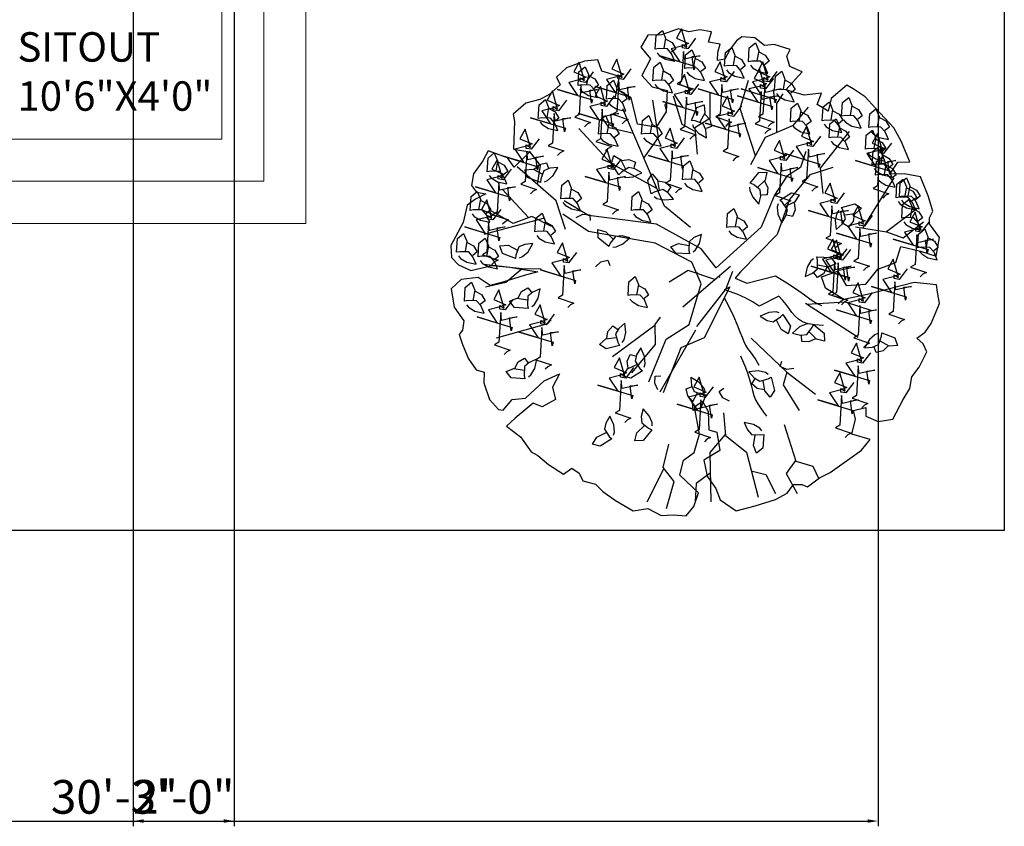
# Model space of a CAD drawing. Units: inches. Extents: x 3394 to 4794, y 965 to 1718.
# Tile 13 of 15: x 4500 to 4734, y 987 to 1179. Entities that reach past the tile are written whole.
import ezdxf

# ---------------------------------------------------------------- set-up
doc = ezdxf.new("R2010")
doc.units = ezdxf.units.IN
for name, color, linetype, lineweight in [('A-ANNO-DIMS', 2, 'Continuous', 13), ('A-AREA-IDEN', 7, 'Continuous', 18), ('A-FLOR-STRS', 7, 'Continuous', 18), ('C-PROP', 7, 'Continuous', 25), ('CAY', 94, 'Continuous', 13)]:
    doc.layers.add(name, color=color, linetype=linetype, lineweight=lineweight)
doc.layers.add('ARBOL', color=74, linetype='Continuous')
doc.layers.add('TALLO', color=36, linetype='Continuous')
doc.styles.get("Standard").update_dxf_attribs({"font": 'arial.ttf'})
doc.dimstyles.new('ISO-25', dxfattribs={"dimtxt": 8, "dimasz": 2.5, "dimexe": 1.25, "dimexo": 0.625, "dimtad": 1, "dimlunit": 3, "dimtxsty": 'Standard', "dimcen": 2.5, "dimadec": 0, "dimazin": 0, "dimtfac": 1, "dimtmove": 0, "dimatfit": 3, "dimfxl": 1, "dimarcsym": 0})

# ---------------------------------------------------------------- blocks, each defined once
blk = doc.blocks.new('fresno')
at = {"layer": 'ARBOL'}
for p, q in [((2.96, 0.991), (3.575, 1.984)), ((-3.638, 1.194), (-4.164, 1.76)), ((-1.151, -0.932), (-1.99, -1.556)), ((-0.974, -3.757), (-1.31, -4.423))]:
    blk.add_line(p, q, dxfattribs=at)
blk.add_lwpolyline([(0.823, 4.745), (0.566, 4.764), (0.459, 4.687), (0.336, 4.518), (0.233, 4.322), (0.087, 4.298), (0.091, 4.464), (0.14, 4.621), (-0.09, 4.659), (-0.033, 4.863), (-0.264, 4.901), (-0.483, 4.866), (-0.686, 4.924), (-1.021, 4.801), (-1.288, 4.8), (-1.431, 4.563), (-1.234, 4.327), (-1.406, 4), (-1.205, 3.778), (-0.909, 3.705), (-0.931, 3.283), (-1.122, 2.983), (-1.491, 3.043), (-1.619, 3.562), (-1.9, 3.727), (-1.851, 3.982), (-2.197, 4.084), (-2.278, 4.31), (-2.543, 4.283), (-2.896, 4.152), (-3.091, 3.971), (-3.022, 3.817), (-3.244, 3.617), (-3.424, 3.528), (-3.697, 3.455), (-3.946, 3.236), (-3.922, 3.09), (-3.94, 2.548), (-3.617, 2.495), (-3.927, 2.19), (-4.062, 2.379), (-4.443, 2.512), (-4.546, 2.316), (-4.73, 2.062), (-4.767, 1.832), (-4.671, 1.698), (-4.486, 1.667), (-4.693, 1.559), (-4.854, 1.444), (-4.934, 1.102), (-5.037, 0.905), (-5.175, 0.644), (-5.166, 0.406), (-5.024, 0.264), (-4.781, 0.153), (-4.363, 0.249), (-4.014, 0.215), (-3.783, 0.177), (-3.46, 0.124), (-3.733, 0.051), (-4.132, -0.073), (-4.404, -0.146), (-4.639, 0.011), (-4.977, -0.028), (-5.172, -0.209), (-5.113, -0.574), (-4.921, -0.843), (-4.951, -1.027), (-5.012, -1.112), (-4.95, -1.311), (-4.83, -1.592), (-4.676, -1.807), (-4.518, -1.856), (-4.529, -2.068), (-4.417, -2.394), (-4.236, -2.59), (-4.143, -2.605), (-3.967, -2.397), (-3.703, -2.37), (-3.339, -2.027), (-3.032, -1.889), (-3.169, -2.15), (-3.115, -2.396), (-3.376, -2.542), (-3.552, -2.466), (-3.909, -2.762), (-4.077, -2.924), (-3.804, -3.135), (-3.592, -3.43), (-3.461, -3.499), (-3.253, -3.676), (-2.953, -3.867), (-2.792, -3.752), (-2.642, -3.848), (-2.572, -4.001), (-2.323, -4.066), (-2.18, -4.208), (-1.926, -4.392), (-1.58, -4.591), (-1.288, -4.545), (-1.027, -4.683), (-0.788, -4.675), (-0.531, -4.693), (-0.382, -4.505), (-0.29, -4.236), (-0.66, -3.891), (-0.588, -3.595), (-0.374, -3.441), (-0.267, -3.079), (-0.368, -2.541), (-0.208, -2.426), (-0.099, -2.633), (-0.087, -2.991), (0.071, -3.04), (0.129, -3.405), (-0.185, -3.59), (-0.119, -3.909), (0.055, -4.151), (0.136, -4.377), (0.456, -4.596), (0.828, -4.491), (1.227, -4.368), (1.461, -4.241), (1.583, -4.071), (1.748, -4.075), (1.86, -4.117), (2.101, -3.944), (2.308, -3.836), (2.925, -3.393), (3.101, -3.185), (2.74, -3.078), (2.812, -2.782), (2.769, -2.61), (3.015, -2.555), (3.012, -2.721), (3.254, -2.832), (3.546, -2.785), (3.752, -2.393), (3.882, -2.177), (3.92, -1.947), (4.069, -1.758), (4.214, -1.451), (4.144, -1.297), (4.021, -1.182), (4.182, -1.067), (4.304, -0.897), (4.464, -0.497), (4.429, -0.279), (4.406, -0.133), (3.964, -0.083), (3.074, -0.315), (2.582, -0.424), (2.217, -0.197), (2.136, 0.029), (2.462, 0.141), (2.628, -0.147), (3.012, -0.116), (3.249, 0.177), (3.602, 0.308), (3.701, 0.623), (4.089, 0.535), (4.404, 0.436), (4.464, 0.805), (4.272, 1.074), (4.267, 1.193), (4.336, 1.324), (4.243, 1.623), (4.092, 2.003), (3.769, 2.057), (3.485, 2.056), (3.642, 2.291), (3.88, 2.299), (3.71, 2.706), (3.563, 2.967), (3.201, 3.358), (3.001, 3.581), (2.766, 3.738), (2.635, 3.807), (2.332, 3.549), (2.268, 3.299), (2.052, 3.429), (2.136, 3.652), (1.798, 3.613), (1.437, 3.72), (1.755, 4.071), (1.513, 4.182), (1.451, 4.381), (1.519, 4.512), (1.204, 4.611), (1.012, 4.596)], close=True, dxfattribs=at)
for points in [[(-1.104, 4.45), (-1.063, 4.399), (-0.939, 4.325), (-0.757, 4.285), (-0.82, 4.431), (-0.903, 4.527), (-1.075, 4.533), (-1.143, 4.521), (-1.126, 4.792), (-1.002, 4.891), (-0.939, 4.738), (-0.975, 4.535)], [(-0.346, 4.735), (-0.501, 4.528), (-0.605, 4.545), (-0.605, 4.614), (-0.519, 4.563), (-0.622, 4.925), (-0.726, 4.735), (-0.484, 4.632), (-0.622, 4.58), (-0.829, 4.528), (-0.657, 4.27), (-1.053, 4.39), (-0.363, 4.183), (-0.381, 4.114), (-0.415, 4.373), (-0.26, 4.39), (-0.57, 4.321), (-0.588, 4.476), (-0.622, 3.89), (-0.708, 3.839), (-0.398, 3.735), (-0.467, 3.701), (-0.519, 3.649)], [(-0.935, 4.717), (-0.809, 4.65), (-0.736, 4.529), (-0.824, 4.459)], [(-0.521, 4.069), (-0.48, 4.018), (-0.356, 3.944), (-0.174, 3.904), (-0.237, 4.051), (-0.32, 4.146), (-0.492, 4.152), (-0.56, 4.14), (-0.543, 4.411), (-0.419, 4.511), (-0.356, 4.357), (-0.392, 4.154)], [(0.263, 4.114), (0.304, 4.063), (0.429, 3.989), (0.611, 3.948), (0.547, 4.095), (0.465, 4.191), (0.293, 4.197), (0.225, 4.185), (0.242, 4.456), (0.366, 4.555), (0.428, 4.402), (0.393, 4.199)], [(0.734, 4.203), (0.775, 4.152), (0.9, 4.078), (1.082, 4.038), (1.018, 4.185), (0.936, 4.281), (0.763, 4.287), (0.696, 4.274), (0.712, 4.546), (0.837, 4.645), (0.899, 4.491), (0.863, 4.289)], [(0.904, 4.471), (1.029, 4.404), (1.102, 4.282), (1.015, 4.212)], [(-1.623, 4.132), (-1.778, 3.925), (-1.882, 3.942), (-1.882, 4.011), (-1.795, 3.959), (-1.899, 4.321), (-2.002, 4.132), (-1.761, 4.028), (-1.899, 3.977), (-2.106, 3.925), (-1.933, 3.666), (-2.33, 3.787), (-1.64, 3.58), (-1.657, 3.511), (-1.692, 3.77), (-1.537, 3.787), (-1.847, 3.718), (-1.864, 3.873), (-1.899, 3.287), (-1.985, 3.235), (-1.675, 3.132), (-1.744, 3.097), (-1.795, 3.046)], [(-0.352, 4.337), (-0.226, 4.269), (-0.153, 4.148), (-0.241, 4.078)], [(0.433, 4.381), (0.558, 4.314), (0.631, 4.193), (0.544, 4.122)], [(-2.368, 4.073), (-2.523, 3.866), (-2.627, 3.883), (-2.627, 3.952), (-2.541, 3.9), (-2.644, 4.262), (-2.748, 4.073), (-2.506, 3.969), (-2.644, 3.918), (-2.851, 3.866), (-2.679, 3.607), (-3.075, 3.728), (-2.385, 3.521), (-2.403, 3.452), (-2.437, 3.711), (-2.282, 3.728), (-2.592, 3.659), (-2.61, 3.814), (-2.644, 3.228), (-2.73, 3.176), (-2.42, 3.073), (-2.489, 3.038), (-2.541, 2.987)], [(-2.629, 3.733), (-2.588, 3.682), (-2.463, 3.608), (-2.281, 3.568), (-2.345, 3.715), (-2.427, 3.81), (-2.6, 3.816), (-2.667, 3.804), (-2.651, 4.075), (-2.526, 4.175), (-2.464, 4.021), (-2.5, 3.818)], [(-1.149, 3.822), (-1.108, 3.771), (-0.983, 3.697), (-0.802, 3.657), (-0.865, 3.804), (-0.948, 3.9), (-1.12, 3.906), (-1.188, 3.893), (-1.171, 4.165), (-1.047, 4.264), (-0.984, 4.111), (-1.02, 3.908)], [(-0.98, 4.09), (-0.854, 4.023), (-0.781, 3.901), (-0.869, 3.831)], [(0.413, 4.08), (0.258, 3.873), (0.154, 3.89), (0.154, 3.959), (0.241, 3.908), (0.137, 4.27), (0.034, 4.08), (0.275, 3.977), (0.137, 3.925), (-0.07, 3.873), (0.103, 3.614), (-0.294, 3.735), (0.396, 3.528), (0.379, 3.459), (0.344, 3.718), (0.499, 3.735), (0.189, 3.666), (0.172, 3.821), (0.137, 3.235), (0.051, 3.183), (0.361, 3.08), (0.292, 3.046), (0.241, 2.994)], [(1.189, 3.942), (1.034, 3.735), (0.931, 3.752), (0.931, 3.821), (1.017, 3.77), (0.913, 4.132), (0.81, 3.942), (1.051, 3.839), (0.913, 3.787), (0.706, 3.735), (0.879, 3.477), (0.482, 3.597), (1.172, 3.39), (1.155, 3.321), (1.12, 3.58), (1.276, 3.597), (0.965, 3.528), (0.948, 3.683), (0.913, 3.097), (0.827, 3.046), (1.138, 2.942), (1.069, 2.908), (1.017, 2.856)], [(1.259, 4.08), (1.103, 3.873), (1, 3.89), (1, 3.959), (1.086, 3.908), (0.982, 4.27), (0.879, 4.08), (1.12, 3.977), (0.982, 3.925), (0.775, 3.873), (0.948, 3.614), (0.551, 3.735), (1.241, 3.528), (1.224, 3.459), (1.189, 3.718), (1.345, 3.735), (1.034, 3.666), (1.017, 3.821), (0.982, 3.235), (0.896, 3.183), (1.207, 3.08), (1.138, 3.046), (1.086, 2.994)], [(1.25, 3.643), (1.291, 3.592), (1.416, 3.518), (1.597, 3.478), (1.534, 3.625), (1.451, 3.721), (1.279, 3.727), (1.211, 3.714), (1.228, 3.985), (1.352, 4.085), (1.415, 3.931), (1.379, 3.729)], [(-2.459, 4), (-2.334, 3.933), (-2.261, 3.812), (-2.348, 3.742)], [(-2.068, 3.464), (-2.027, 3.413), (-1.903, 3.339), (-1.721, 3.299), (-1.784, 3.446), (-1.867, 3.542), (-2.039, 3.547), (-2.107, 3.535), (-2.09, 3.806), (-1.966, 3.906), (-1.903, 3.752), (-1.939, 3.55)], [(-0.287, 3.833), (-0.442, 3.626), (-0.546, 3.643), (-0.546, 3.712), (-0.46, 3.661), (-0.563, 4.023), (-0.667, 3.833), (-0.425, 3.73), (-0.563, 3.678), (-0.77, 3.626), (-0.598, 3.367), (-0.995, 3.488), (-0.304, 3.281), (-0.322, 3.212), (-0.356, 3.471), (-0.201, 3.488), (-0.511, 3.419), (-0.529, 3.574), (-0.563, 2.988), (-0.649, 2.936), (-0.339, 2.833), (-0.408, 2.799), (-0.46, 2.747)], [(0.837, 2.414), (0.533, 3.352), (0.697, 3.906)], [(1.419, 3.911), (1.545, 3.844), (1.618, 3.722), (1.53, 3.652)], [(-2.898, 3.511), (-3.053, 3.304), (-3.157, 3.321), (-3.157, 3.39), (-3.071, 3.339), (-3.174, 3.701), (-3.278, 3.511), (-3.036, 3.408), (-3.174, 3.356), (-3.381, 3.304), (-3.209, 3.046), (-3.605, 3.166), (-2.915, 2.959), (-2.932, 2.89), (-2.967, 3.149), (-2.812, 3.166), (-3.122, 3.097), (-3.14, 3.253), (-3.174, 2.666), (-3.26, 2.615), (-2.95, 2.511), (-3.019, 2.477), (-3.071, 2.425)], [(-1.951, 3.597), (-2.106, 3.39), (-2.209, 3.408), (-2.209, 3.477), (-2.123, 3.425), (-2.227, 3.787), (-2.33, 3.597), (-2.089, 3.494), (-2.227, 3.442), (-2.434, 3.39), (-2.261, 3.132), (-2.658, 3.252), (-1.968, 3.046), (-1.985, 2.977), (-2.02, 3.235), (-1.864, 3.252), (-2.175, 3.183), (-2.192, 3.339), (-2.227, 2.752), (-2.313, 2.701), (-2.002, 2.597), (-2.071, 2.563), (-2.123, 2.511)], [(-1.899, 3.732), (-1.773, 3.664), (-1.7, 3.543), (-1.788, 3.473)], [(-3.413, 3.083), (-3.373, 3.032), (-3.248, 2.958), (-3.066, 2.918), (-3.129, 3.065), (-3.212, 3.161), (-3.384, 3.167), (-3.452, 3.154), (-3.435, 3.425), (-3.311, 3.525), (-3.248, 3.371), (-3.284, 3.169)], [(-1.367, 2.367), (-1.081, 2.78), (-1.193, 3.514)], [(-0.358, 2.895), (-0.615, 3.037), (-0.783, 3.596)], [(-0.063, 3.671), (-0.069, 3.151), (-0.364, 2.965), (-0.319, 2.449)], [(0.558, 3.402), (0.403, 3.195), (0.299, 3.212), (0.299, 3.281), (0.386, 3.23), (0.282, 3.592), (0.179, 3.402), (0.42, 3.299), (0.282, 3.247), (0.075, 3.195), (0.248, 2.936), (-0.149, 3.057), (0.541, 2.85), (0.524, 2.781), (0.489, 3.04), (0.644, 3.057), (0.334, 2.988), (0.317, 3.143), (0.282, 2.557), (0.196, 2.505), (0.506, 2.402), (0.437, 2.368), (0.386, 2.316)], [(1.259, 2.882), (1.254, 3.446), (1.381, 3.636)], [(2.573, 3.128), (2.613, 3.077), (2.738, 3.003), (2.92, 2.963), (2.857, 3.11), (2.774, 3.205), (2.602, 3.211), (2.534, 3.199), (2.551, 3.47), (2.675, 3.57), (2.738, 3.416), (2.702, 3.214)], [(-3.244, 3.351), (-3.118, 3.284), (-3.045, 3.162), (-3.133, 3.092)], [(-0.448, 1), (-0.961, 1.419), (-1.784, 3.341)], [(-0.923, 3.449), (-0.951, 3.425), (-0.93, 3.313)], [(-0.41, 3.035), (-0.387, 2.974), (-0.291, 2.865), (-0.131, 2.771), (-0.146, 2.93), (-0.195, 3.047), (-0.357, 3.106), (-0.425, 3.115), (-0.325, 3.368), (-0.176, 3.424), (-0.164, 3.258), (-0.261, 3.077)], [(0.746, 2.242), (1.034, 2.786), (1.584, 3.019), (1.879, 3.374)], [(1.564, 3.016), (1.605, 2.965), (1.729, 2.891), (1.911, 2.851), (1.848, 2.998), (1.765, 3.094), (1.593, 3.099), (1.525, 3.087), (1.542, 3.358), (1.666, 3.458), (1.729, 3.304), (1.693, 3.102)], [(2.191, 3.038), (2.232, 2.987), (2.357, 2.913), (2.539, 2.873), (2.475, 3.02), (2.393, 3.116), (2.221, 3.122), (2.153, 3.109), (2.17, 3.381), (2.294, 3.48), (2.356, 3.326), (2.321, 3.124)], [(2.361, 3.306), (2.486, 3.239), (2.559, 3.117), (2.472, 3.047)], [(2.742, 3.396), (2.868, 3.328), (2.941, 3.207), (2.853, 3.137)], [(3.111, 2.904), (3.152, 2.853), (3.276, 2.779), (3.458, 2.739), (3.395, 2.886), (3.312, 2.981), (3.14, 2.987), (3.072, 2.975), (3.089, 3.246), (3.213, 3.346), (3.276, 3.192), (3.24, 2.99)], [(-2.225, 2.77), (-2.184, 2.718), (-2.06, 2.645), (-1.878, 2.604), (-1.941, 2.751), (-2.024, 2.847), (-2.196, 2.853), (-2.264, 2.84), (-2.247, 3.112), (-2.123, 3.211), (-2.06, 3.058), (-2.096, 2.855)], [(-1.575, 2.854), (-2.052, 2.969), (-2.2, 3.178)], [(-1.373, 2.77), (-1.332, 2.718), (-1.208, 2.645), (-1.026, 2.604), (-1.089, 2.751), (-1.172, 2.847), (-1.344, 2.853), (-1.412, 2.84), (-1.395, 3.112), (-1.271, 3.211), (-1.208, 3.058), (-1.244, 2.855)], [(-0.166, 3.238), (-0.068, 3.135), (-0.036, 2.997), (-0.141, 2.957)], [(1.733, 3.284), (1.859, 3.216), (1.932, 3.095), (1.844, 3.025)], [(2.326, 2.702), (2.367, 2.651), (2.492, 2.577), (2.673, 2.537), (2.61, 2.684), (2.527, 2.78), (2.355, 2.786), (2.287, 2.773), (2.304, 3.045), (2.428, 3.144), (2.491, 2.99), (2.455, 2.788)], [(3.28, 3.172), (3.406, 3.104), (3.479, 2.983), (3.391, 2.913)], [(-3.434, 2.752), (-3.59, 2.546), (-3.693, 2.563), (-3.693, 2.632), (-3.607, 2.58), (-3.71, 2.942), (-3.814, 2.752), (-3.572, 2.649), (-3.71, 2.597), (-3.917, 2.546), (-3.745, 2.287), (-4.142, 2.408), (-3.452, 2.201), (-3.469, 2.132), (-3.503, 2.39), (-3.348, 2.408), (-3.659, 2.339), (-3.676, 2.494), (-3.71, 1.908), (-3.797, 1.856), (-3.486, 1.753), (-3.555, 1.718), (-3.607, 1.666)], [(-1.112, 1.773), (-2.014, 2.265), (-2.654, 2.957)], [(-2.056, 3.037), (-1.93, 2.97), (-1.857, 2.849), (-1.945, 2.778)], [(-0.57, 2.77), (-0.726, 2.563), (-0.829, 2.58), (-0.829, 2.649), (-0.743, 2.597), (-0.846, 2.959), (-0.95, 2.77), (-0.708, 2.666), (-0.846, 2.615), (-1.053, 2.563), (-0.881, 2.304), (-1.278, 2.425), (-0.588, 2.218), (-0.605, 2.149), (-0.639, 2.408), (-0.484, 2.425), (-0.795, 2.356), (-0.812, 2.511), (-0.846, 1.925), (-0.933, 1.873), (-0.622, 1.77), (-0.691, 1.735), (-0.743, 1.684)], [(-1.204, 3.037), (-1.078, 2.97), (-1.005, 2.849), (-1.093, 2.778)], [(2.121, 2.804), (1.966, 2.597), (1.862, 2.615), (1.862, 2.683), (1.949, 2.632), (1.845, 2.994), (1.742, 2.804), (1.983, 2.701), (1.845, 2.649), (1.638, 2.597), (1.811, 2.339), (1.414, 2.459), (2.104, 2.252), (2.087, 2.184), (2.052, 2.442), (2.207, 2.459), (1.897, 2.39), (1.88, 2.546), (1.845, 1.959), (1.759, 1.908), (2.069, 1.804), (2, 1.77), (1.949, 1.718)], [(2.495, 2.97), (2.621, 2.903), (2.694, 2.781), (2.606, 2.711)], [(3.043, 2.478), (3.084, 2.427), (3.209, 2.353), (3.391, 2.313), (3.327, 2.46), (3.245, 2.556), (3.073, 2.562), (3.005, 2.549), (3.022, 2.82), (3.146, 2.92), (3.208, 2.766), (3.173, 2.564)], [(2.171, 1.674), (2.121, 2.172), (2.689, 2.898)], [(3.519, 2.666), (3.363, 2.459), (3.26, 2.477), (3.26, 2.546), (3.346, 2.494), (3.243, 2.856), (3.139, 2.666), (3.381, 2.563), (3.243, 2.511), (3.036, 2.459), (3.208, 2.201), (2.811, 2.321), (3.501, 2.115), (3.484, 2.046), (3.45, 2.304), (3.605, 2.321), (3.294, 2.252), (3.277, 2.408), (3.243, 1.821), (3.156, 1.77), (3.467, 1.666), (3.398, 1.632), (3.346, 1.58)], [(3.213, 2.746), (3.338, 2.679), (3.411, 2.557), (3.324, 2.487)], [(-1.817, 2.351), (-1.972, 2.144), (-2.075, 2.162), (-2.075, 2.231), (-1.989, 2.179), (-2.093, 2.541), (-2.196, 2.351), (-1.955, 2.248), (-2.093, 2.196), (-2.3, 2.144), (-2.127, 1.886), (-2.524, 2.006), (-1.834, 1.8), (-1.851, 1.731), (-1.886, 1.989), (-1.73, 2.006), (-2.041, 1.937), (-2.058, 2.093), (-2.093, 1.506), (-2.179, 1.455), (-1.868, 1.351), (-1.937, 1.317), (-1.989, 1.265)], [(1.586, 2.528), (1.431, 2.321), (1.327, 2.339), (1.327, 2.408), (1.414, 2.356), (1.31, 2.718), (1.207, 2.528), (1.448, 2.425), (1.31, 2.373), (1.103, 2.321), (1.276, 2.063), (0.879, 2.184), (1.569, 1.977), (1.552, 1.908), (1.517, 2.166), (1.673, 2.184), (1.362, 2.115), (1.345, 2.27), (1.31, 1.684), (1.224, 1.632), (1.535, 1.528), (1.466, 1.494), (1.414, 1.442)], [(3.178, 2.165), (3.219, 2.113), (3.344, 2.04), (3.525, 1.999), (3.462, 2.146), (3.379, 2.242), (3.207, 2.248), (3.139, 2.236), (3.156, 2.507), (3.28, 2.606), (3.343, 2.453), (3.307, 2.25)], [(-3.986, 2.149), (-4.142, 1.942), (-4.245, 1.959), (-4.245, 2.028), (-4.159, 1.977), (-4.262, 2.339), (-4.366, 2.149), (-4.124, 2.046), (-4.262, 1.994), (-4.47, 1.942), (-4.297, 1.684), (-4.694, 1.804), (-4.004, 1.597), (-4.021, 1.528), (-4.055, 1.787), (-3.9, 1.804), (-4.211, 1.735), (-4.228, 1.89), (-4.262, 1.304), (-4.349, 1.253), (-4.038, 1.149), (-4.107, 1.115), (-4.159, 1.063)], [(-4.422, 2.03), (-4.381, 1.979), (-4.257, 1.905), (-4.075, 1.865), (-4.138, 2.012), (-4.221, 2.108), (-4.393, 2.114), (-4.461, 2.101), (-4.444, 2.372), (-4.32, 2.472), (-4.257, 2.318), (-4.293, 2.116)], [(-3.468, 1.85), (-3.409, 2.222), (-3.628, 2.505)], [(-1.786, 2.007), (-1.722, 1.99), (-1.578, 2.003), (-1.407, 2.078), (-1.545, 2.159), (-1.668, 2.188), (-1.811, 2.092), (-1.859, 2.042), (-2.004, 2.271), (-1.962, 2.425), (-1.821, 2.337), (-1.731, 2.152)], [(-1.806, 2.323), (-1.665, 2.343), (-1.534, 2.287), (-1.564, 2.179)], [(3.245, 1.963), (3.286, 1.912), (3.411, 1.838), (3.593, 1.798), (3.529, 1.945), (3.447, 2.041), (3.274, 2.046), (3.206, 2.034), (3.223, 2.305), (3.347, 2.405), (3.41, 2.251), (3.374, 2.049)], [(3.347, 2.432), (3.473, 2.365), (3.546, 2.244), (3.458, 2.173)], [(-4.253, 2.298), (-4.127, 2.231), (-4.054, 2.109), (-4.142, 2.039)], [(-2.916, 0.958), (-3.096, 1.528), (-3.871, 2.197)], [(-3.331, 1.905), (-3.269, 1.928), (-3.161, 2.024), (-3.066, 2.184), (-3.226, 2.169), (-3.342, 2.121), (-3.401, 1.958), (-3.41, 1.89), (-3.663, 1.99), (-3.719, 2.139), (-3.554, 2.151), (-3.372, 2.054)], [(-3.533, 2.149), (-3.43, 2.247), (-3.292, 2.279), (-3.252, 2.174)], [(-0.566, 1.873), (-0.525, 1.822), (-0.4, 1.748), (-0.219, 1.708), (-0.282, 1.855), (-0.365, 1.951), (-0.537, 1.957), (-0.605, 1.944), (-0.588, 2.216), (-0.464, 2.315), (-0.401, 2.162), (-0.437, 1.959)], [(-0.397, 2.141), (-0.271, 2.074), (-0.198, 1.952), (-0.286, 1.882)], [(3.415, 2.231), (3.54, 2.163), (3.613, 2.042), (3.525, 1.972)], [(-1.164, 1.612), (-1.109, 1.576), (-0.967, 1.544), (-0.782, 1.562), (-0.888, 1.682), (-0.996, 1.748), (-1.162, 1.7), (-1.222, 1.667), (-1.29, 1.93), (-1.203, 2.063), (-1.096, 1.937), (-1.067, 1.733)], [(0.72, 1.798), (0.723, 1.733), (0.781, 1.6), (0.904, 1.46), (0.939, 1.616), (0.929, 1.742), (0.793, 1.848), (0.73, 1.878), (0.904, 2.088), (1.062, 2.095), (1.023, 1.934), (0.875, 1.791)], [(3.649, 1.515), (3.69, 1.464), (3.814, 1.39), (3.996, 1.35), (3.933, 1.497), (3.85, 1.592), (3.678, 1.598), (3.61, 1.586), (3.627, 1.857), (3.751, 1.957), (3.814, 1.803), (3.778, 1.601)], [(3.716, 1.537), (3.757, 1.486), (3.882, 1.412), (4.063, 1.372), (4, 1.519), (3.917, 1.615), (3.745, 1.621), (3.677, 1.608), (3.694, 1.88), (3.818, 1.979), (3.881, 1.825), (3.845, 1.623)], [(-2.965, 1.493), (-2.924, 1.441), (-2.799, 1.368), (-2.618, 1.327), (-2.681, 1.474), (-2.764, 1.57), (-2.936, 1.576), (-3.004, 1.564), (-2.987, 1.835), (-2.863, 1.934), (-2.8, 1.781), (-2.836, 1.578)], [(-2.796, 1.76), (-2.67, 1.693), (-2.597, 1.572), (-2.685, 1.501)], [(-1.085, 1.919), (-0.945, 1.893), (-0.838, 1.801), (-0.9, 1.707)], [(1.014, 1.915), (1.077, 1.787), (1.064, 1.646), (0.952, 1.64)], [(2.587, 1.684), (2.432, 1.477), (2.328, 1.494), (2.328, 1.563), (2.414, 1.511), (2.311, 1.873), (2.207, 1.684), (2.449, 1.58), (2.311, 1.528), (2.104, 1.477), (2.276, 1.218), (1.88, 1.339), (2.57, 1.132), (2.552, 1.063), (2.518, 1.321), (2.673, 1.339), (2.363, 1.27), (2.345, 1.425), (2.311, 0.839), (2.225, 0.787), (2.535, 0.684), (2.466, 0.649), (2.414, 0.597)], [(3.818, 1.783), (3.944, 1.715), (4.017, 1.594), (3.929, 1.524)], [(3.885, 1.805), (4.011, 1.738), (4.084, 1.616), (3.996, 1.546)], [(-4.759, 1.269), (-4.718, 1.217), (-4.593, 1.144), (-4.411, 1.103), (-4.475, 1.25), (-4.557, 1.346), (-4.729, 1.352), (-4.797, 1.339), (-4.78, 1.611), (-4.656, 1.71), (-4.594, 1.557), (-4.629, 1.354)], [(-1.575, 1.269), (-1.534, 1.217), (-1.409, 1.144), (-1.228, 1.103), (-1.291, 1.25), (-1.373, 1.346), (-1.546, 1.352), (-1.614, 1.339), (-1.597, 1.611), (-1.473, 1.71), (-1.41, 1.557), (-1.446, 1.354)], [(1.283, 1.469), (1.266, 1.405), (1.279, 1.261), (1.354, 1.09), (1.435, 1.228), (1.464, 1.351), (1.368, 1.494), (1.318, 1.542), (1.547, 1.687), (1.7, 1.645), (1.613, 1.504), (1.428, 1.414)], [(-4.193, 1.356), (-4.349, 1.149), (-4.452, 1.166), (-4.452, 1.235), (-4.366, 1.184), (-4.469, 1.546), (-4.573, 1.356), (-4.331, 1.253), (-4.469, 1.201), (-4.677, 1.149), (-4.504, 0.89), (-4.901, 1.011), (-4.211, 0.804), (-4.228, 0.735), (-4.262, 0.994), (-4.107, 1.011), (-4.418, 0.942), (-4.435, 1.097), (-4.469, 0.511), (-4.556, 0.459), (-4.245, 0.356), (-4.314, 0.322), (-4.366, 0.27)], [(-4.589, 1.536), (-4.464, 1.469), (-4.391, 1.348), (-4.478, 1.277)], [(-1.406, 1.536), (-1.28, 1.469), (-1.207, 1.348), (-1.295, 1.277)], [(0.308, 0.933), (0.349, 0.881), (0.474, 0.807), (0.656, 0.767), (0.592, 0.914), (0.51, 1.01), (0.337, 1.016), (0.27, 1.003), (0.286, 1.275), (0.411, 1.374), (0.473, 1.221), (0.437, 1.018)], [(1.599, 1.489), (1.618, 1.348), (1.563, 1.217), (1.455, 1.247)], [(2.479, 1.34), (2.443, 1.285), (2.411, 1.143), (2.429, 0.958), (2.549, 1.064), (2.615, 1.172), (2.567, 1.338), (2.534, 1.398), (2.797, 1.466), (2.93, 1.379), (2.804, 1.272), (2.6, 1.243)], [(3.139, 1.235), (2.984, 1.028), (2.88, 1.046), (2.88, 1.115), (2.967, 1.063), (2.863, 1.425), (2.759, 1.235), (3.001, 1.132), (2.863, 1.08), (2.656, 1.028), (2.828, 0.77), (2.432, 0.891), (3.122, 0.684), (3.105, 0.615), (3.07, 0.873), (3.225, 0.891), (2.915, 0.822), (2.897, 0.977), (2.863, 0.391), (2.777, 0.339), (3.087, 0.235), (3.018, 0.201), (2.967, 0.149)], [(3.761, 1.112), (3.802, 1.061), (3.926, 0.987), (4.108, 0.947), (4.045, 1.093), (3.962, 1.189), (3.79, 1.195), (3.722, 1.183), (3.739, 1.454), (3.863, 1.553), (3.926, 1.4), (3.89, 1.197)], [(3.93, 1.379), (4.056, 1.312), (4.129, 1.191), (4.041, 1.121)], [(-3.354, 1.176), (-4.529, 0.864)], [(-3.192, 1.017), (-3.578, 1.215), (-3.949, 1.081), (-4.398, 1.339)], [(-3.481, 0.843), (-3.44, 0.792), (-3.315, 0.718), (-3.133, 0.678), (-3.197, 0.825), (-3.279, 0.92), (-3.451, 0.926), (-3.519, 0.914), (-3.502, 1.185), (-3.378, 1.285), (-3.316, 1.131), (-3.351, 0.928)], [(-2.703, 1.201), (-2.575, 1.263), (-2.433, 1.251), (-2.428, 1.139)], [(0.478, 1.2), (0.603, 1.133), (0.676, 1.011), (0.589, 0.941)], [(2.786, 1.261), (2.76, 1.121), (2.668, 1.014), (2.574, 1.076)], [(4.01, 1.36), (3.422, 0.918)], [(4.26, 1.115), (4.105, 0.908), (4.002, 0.925), (4.002, 0.994), (4.088, 0.942), (3.984, 1.304), (3.881, 1.115), (4.122, 1.011), (3.984, 0.959), (3.777, 0.908), (3.95, 0.649), (3.553, 0.77), (4.243, 0.563), (4.226, 0.494), (4.191, 0.753), (4.347, 0.77), (4.036, 0.701), (4.019, 0.856), (3.984, 0.27), (3.898, 0.218), (4.209, 0.115), (4.14, 0.08), (4.088, 0.029)], [(-3.311, 1.111), (-3.186, 1.043), (-3.113, 0.922), (-3.2, 0.852)], [(2.808, 1.015), (3.422, 0.918), (3.422, 0.918), (3.748, 0.794), (4.154, 1.111)], [(-5.028, 0.44), (-4.987, 0.388), (-4.862, 0.315), (-4.68, 0.274), (-4.744, 0.421), (-4.826, 0.517), (-4.998, 0.523), (-5.066, 0.511), (-5.049, 0.782), (-4.925, 0.881), (-4.863, 0.728), (-4.898, 0.525)], [(-4.602, 0.35), (-4.561, 0.299), (-4.436, 0.225), (-4.254, 0.185), (-4.318, 0.332), (-4.4, 0.428), (-4.572, 0.433), (-4.64, 0.421), (-4.623, 0.692), (-4.499, 0.792), (-4.437, 0.638), (-4.472, 0.436)], [(-1.981, 0.615), (-1.915, 0.618), (-1.782, 0.676), (-1.643, 0.799), (-1.799, 0.834), (-1.925, 0.824), (-2.031, 0.688), (-2.061, 0.626), (-2.27, 0.799), (-2.278, 0.958), (-2.117, 0.918), (-1.974, 0.77)], [(-0.397, 0.517), (-0.346, 0.557), (-0.272, 0.682), (-0.232, 0.864), (-0.379, 0.801), (-0.474, 0.718), (-0.48, 0.546), (-0.468, 0.478), (-0.739, 0.495), (-0.838, 0.619), (-0.685, 0.682), (-0.482, 0.646)], [(4.075, 0.529), (4.116, 0.478), (4.24, 0.404), (4.422, 0.364), (4.359, 0.511), (4.276, 0.607), (4.104, 0.613), (4.036, 0.6), (4.053, 0.871), (4.177, 0.971), (4.24, 0.817), (4.204, 0.615)], [(4.244, 0.797), (4.37, 0.73), (4.443, 0.608), (4.355, 0.538)], [(-4.858, 0.707), (-4.733, 0.64), (-4.66, 0.519), (-4.747, 0.448)], [(-4.432, 0.618), (-4.307, 0.55), (-4.234, 0.429), (-4.321, 0.359)], [(-3.824, 0.404), (-3.763, 0.427), (-3.654, 0.523), (-3.559, 0.683), (-3.719, 0.668), (-3.835, 0.62), (-3.894, 0.457), (-3.903, 0.389), (-4.156, 0.489), (-4.212, 0.638), (-4.047, 0.65), (-3.865, 0.553)], [(-2.698, 0.509), (-2.854, 0.302), (-2.957, 0.319), (-2.957, 0.388), (-2.871, 0.336), (-2.974, 0.698), (-3.078, 0.509), (-2.836, 0.405), (-2.974, 0.353), (-3.182, 0.302), (-3.009, 0.043), (-3.406, 0.164), (-2.716, -0.043), (-2.733, -0.112), (-2.767, 0.147), (-2.612, 0.164), (-2.923, 0.095), (-2.94, 0.25), (-2.974, -0.336), (-3.061, -0.388), (-2.75, -0.491), (-2.819, -0.526), (-2.871, -0.577)], [(2.639, 0.58), (2.483, 0.373), (2.38, 0.391), (2.38, 0.46), (2.466, 0.408), (2.363, 0.77), (2.259, 0.58), (2.501, 0.477), (2.363, 0.425), (2.156, 0.373), (2.328, 0.115), (1.931, 0.235), (2.621, 0.029), (2.604, -0.04), (2.57, 0.218), (2.725, 0.235), (2.414, 0.166), (2.397, 0.322), (2.363, -0.265), (2.276, -0.316), (2.587, -0.42), (2.518, -0.454), (2.466, -0.506)], [(2.708, 0.563), (2.552, 0.356), (2.449, 0.373), (2.449, 0.442), (2.535, 0.391), (2.432, 0.753), (2.328, 0.563), (2.57, 0.46), (2.432, 0.408), (2.225, 0.356), (2.397, 0.097), (2, 0.218), (2.69, 0.011), (2.673, -0.058), (2.639, 0.201), (2.794, 0.218), (2.483, 0.149), (2.466, 0.304), (2.432, -0.282), (2.345, -0.334), (2.656, -0.437), (2.587, -0.471), (2.535, -0.523)], [(1.978, 0.384), (1.927, 0.343), (1.853, 0.218), (1.813, 0.036), (1.96, 0.1), (2.056, 0.182), (2.061, 0.355), (2.049, 0.422), (2.32, 0.406), (2.42, 0.281), (2.266, 0.219), (2.064, 0.254)], [(-3.394, 0.18), (-3.77, 0.182), (-4.532, 0.27)], [(-2.322, 0.222), (-2.219, 0.321), (-2.081, 0.353), (-2.042, 0.248)], [(-0.596, -0.564), (0.03, -0.026), (0.339, 0.235)], [(2.246, 0.214), (2.178, 0.089), (2.057, 0.016), (1.987, 0.103)], [(3.829, 0.184), (3.674, -0.023), (3.57, -0.006), (3.57, 0.063), (3.657, 0.011), (3.553, 0.373), (3.45, 0.184), (3.691, 0.08), (3.553, 0.029), (3.346, -0.023), (3.519, -0.282), (3.122, -0.161), (3.812, -0.368), (3.795, -0.437), (3.76, -0.178), (3.915, -0.161), (3.605, -0.23), (3.588, -0.075), (3.553, -0.661), (3.467, -0.713), (3.777, -0.816), (3.708, -0.851), (3.657, -0.902)], [(-3.77, 0.182), (-4.09, -0.088), (-4.494, -0.18)], [(-1.642, -0.412), (-1.601, -0.463), (-1.477, -0.537), (-1.295, -0.577), (-1.358, -0.43), (-1.441, -0.334), (-1.613, -0.328), (-1.681, -0.341), (-1.664, -0.069), (-1.54, 0.03), (-1.477, -0.124), (-1.513, -0.326)], [(0.03, -0.026), (-0.491, 0.154), (-0.871, -0.08)], [(0.38, 0.131), (0.248, -0.21), (-0.33, -0.951)], [(-4.871, -0.524), (-4.83, -0.575), (-4.705, -0.649), (-4.523, -0.689), (-4.587, -0.542), (-4.669, -0.446), (-4.841, -0.44), (-4.909, -0.453), (-4.893, -0.181), (-4.768, -0.082), (-4.706, -0.236), (-4.741, -0.438)], [(-3.848, -0.389), (-3.781, -0.264), (-3.659, -0.191), (-3.589, -0.278)], [(-1.473, -0.144), (-1.347, -0.211), (-1.274, -0.333), (-1.362, -0.403)], [(3.139, -0.282), (2.984, -0.489), (2.88, -0.471), (2.88, -0.402), (2.967, -0.454), (2.863, -0.092), (2.759, -0.282), (3.001, -0.385), (2.863, -0.437), (2.656, -0.489), (2.828, -0.747), (2.432, -0.627), (3.122, -0.834), (3.105, -0.902), (3.07, -0.644), (3.225, -0.627), (2.915, -0.696), (2.897, -0.54), (2.863, -1.127), (2.777, -1.178), (3.087, -1.282), (3.018, -1.316), (2.967, -1.368)], [(-4.701, -0.256), (-4.576, -0.323), (-4.503, -0.445), (-4.59, -0.515)], [(-3.952, -0.42), (-4.107, -0.627), (-4.211, -0.609), (-4.211, -0.54), (-4.124, -0.592), (-4.228, -0.23), (-4.331, -0.42), (-4.09, -0.523), (-4.228, -0.575), (-4.435, -0.627), (-4.262, -0.885), (-4.659, -0.765), (-3.969, -0.971), (-3.986, -1.04), (-4.021, -0.782), (-3.866, -0.765), (-4.176, -0.834), (-4.193, -0.678), (-4.228, -1.265), (-4.314, -1.316), (-4.004, -1.42), (-4.073, -1.454), (-4.124, -1.506)], [(-3.58, -0.559), (-3.529, -0.518), (-3.455, -0.393), (-3.415, -0.211), (-3.562, -0.275), (-3.658, -0.357), (-3.664, -0.53), (-3.651, -0.597), (-3.923, -0.581), (-4.022, -0.456), (-3.868, -0.394), (-3.666, -0.43)], [(-3.141, -0.713), (-3.296, -0.92), (-3.4, -0.902), (-3.4, -0.834), (-3.314, -0.885), (-3.417, -0.523), (-3.521, -0.713), (-3.279, -0.816), (-3.417, -0.868), (-3.624, -0.92), (-3.452, -1.178), (-3.848, -1.058), (-3.158, -1.265), (-3.175, -1.333), (-3.21, -1.075), (-3.055, -1.058), (-3.365, -1.127), (-3.383, -0.971), (-3.417, -1.558), (-3.503, -1.609), (-3.193, -1.713), (-3.262, -1.747), (-3.314, -1.799)], [(1.822, -0.495), (2.859, -1.165)], [(1.846, -0.51), (2.605, -0.469), (3.129, -0.637)], [(-1.047, -0.767), (-1.151, -0.913), (-1.144, -1.307), (-1.61, -1.871)], [(1.304, -0.681), (1.241, -0.664), (1.097, -0.678), (0.926, -0.752), (1.064, -0.833), (1.187, -0.862), (1.33, -0.766), (1.377, -0.716), (1.523, -0.945), (1.481, -1.099), (1.34, -1.011), (1.25, -0.826)], [(-3.195, -0.824), (-3.267, -0.898), (-4.285, -1.185)], [(-1.794, -1.268), (-1.758, -1.214), (-1.726, -1.072), (-1.744, -0.887), (-1.865, -0.993), (-1.93, -1.101), (-1.883, -1.266), (-1.85, -1.327), (-2.113, -1.395), (-2.246, -1.307), (-2.119, -1.2), (-1.916, -1.172)], [(-2.101, -1.19), (-2.076, -1.05), (-1.983, -0.943), (-1.889, -1.004)], [(1.903, -0.903), (1.837, -0.905), (1.704, -0.963), (1.565, -1.086), (1.721, -1.122), (1.847, -1.111), (1.953, -0.975), (1.983, -0.913), (2.192, -1.086), (2.2, -1.245), (2.039, -1.205), (1.896, -1.057)], [(-0.346, -1.024), (-1.05, -2.251)], [(2.02, -1.197), (1.891, -1.259), (1.75, -1.247), (1.745, -1.134)], [(3.253, -1.094), (3.192, -1.117), (3.083, -1.213), (2.988, -1.374), (3.148, -1.359), (3.264, -1.31), (3.323, -1.148), (3.332, -1.079), (3.585, -1.179), (3.641, -1.328), (3.476, -1.34), (3.294, -1.244)], [(0.748, -1.185), (1.452, -1.855), (2.021, -2.292)], [(3.105, -1.471), (2.949, -1.678), (2.846, -1.661), (2.846, -1.592), (2.932, -1.644), (2.829, -1.282), (2.725, -1.471), (2.967, -1.575), (2.829, -1.627), (2.621, -1.678), (2.794, -1.937), (2.397, -1.816), (3.087, -2.023), (3.07, -2.092), (3.036, -1.833), (3.191, -1.816), (2.88, -1.885), (2.863, -1.73), (2.829, -2.316), (2.742, -2.368), (3.053, -2.471), (2.984, -2.506), (2.932, -2.558)], [(3.455, -1.338), (3.352, -1.437), (3.214, -1.469), (3.175, -1.364)], [(-1.361, -1.756), (-1.343, -1.693), (-1.357, -1.548), (-1.431, -1.377), (-1.513, -1.515), (-1.542, -1.638), (-1.445, -1.781), (-1.395, -1.829), (-1.625, -1.974), (-1.778, -1.932), (-1.691, -1.791), (-1.506, -1.701)], [(-1.677, -1.776), (-1.696, -1.635), (-1.641, -1.504), (-1.533, -1.534)], [(-3.648, -1.948), (-3.596, -1.907), (-3.523, -1.782), (-3.482, -1.6), (-3.629, -1.664), (-3.725, -1.746), (-3.731, -1.919), (-3.719, -1.986), (-3.99, -1.97), (-4.089, -1.845), (-3.936, -1.783), (-3.733, -1.819)], [(-3.915, -1.778), (-3.848, -1.653), (-3.727, -1.58), (-3.656, -1.667)], [(-1.571, -1.764), (-1.726, -1.971), (-1.83, -1.954), (-1.83, -1.885), (-1.744, -1.937), (-1.847, -1.575), (-1.951, -1.764), (-1.709, -1.868), (-1.847, -1.92), (-2.054, -1.971), (-1.882, -2.23), (-2.278, -2.109), (-1.588, -2.316), (-1.605, -2.385), (-1.64, -2.127), (-1.485, -2.109), (-1.795, -2.178), (-1.813, -2.023), (-1.847, -2.609), (-1.933, -2.661), (-1.623, -2.764), (-1.692, -2.799), (-1.744, -2.851)], [(1.593, -1.781), (1.452, -1.801), (1.322, -1.746), (1.352, -1.637)], [(-1.092, -2.202), (-1.154, -2.074), (-1.142, -1.933), (-1.03, -1.928)], [(1.086, -1.899), (1.031, -1.863), (0.89, -1.831), (0.704, -1.849), (0.81, -1.969), (0.918, -2.035), (1.084, -1.987), (1.145, -1.954), (1.212, -2.218), (1.125, -2.35), (1.018, -2.224), (0.989, -2.02)], [(1.452, -1.855), (1.379, -2.105), (1.698, -2.609)], [(2.777, -2.058), (2.621, -2.264), (2.518, -2.247), (2.518, -2.178), (2.604, -2.23), (2.501, -1.868), (2.397, -2.058), (2.639, -2.161), (2.501, -2.213), (2.294, -2.264), (2.466, -2.523), (2.069, -2.402), (2.759, -2.609), (2.742, -2.678), (2.708, -2.42), (2.863, -2.402), (2.552, -2.471), (2.535, -2.316), (2.501, -2.902), (2.414, -2.954), (2.725, -3.057), (2.656, -3.092), (2.604, -3.144)], [(-0.001, -2.144), (-0.156, -2.351), (-0.26, -2.333), (-0.26, -2.264), (-0.174, -2.316), (-0.277, -1.954), (-0.381, -2.144), (-0.139, -2.247), (-0.277, -2.299), (-0.484, -2.351), (-0.312, -2.609), (-0.708, -2.489), (-0.018, -2.695), (-0.035, -2.764), (-0.07, -2.506), (0.085, -2.489), (-0.225, -2.558), (-0.243, -2.402), (-0.277, -2.989), (-0.363, -3.04), (-0.053, -3.144), (-0.122, -3.178), (-0.174, -3.23)], [(-0.161, -2.225), (-0.184, -2.163), (-0.28, -2.055), (-0.44, -1.96), (-0.425, -2.12), (-0.376, -2.236), (-0.214, -2.295), (-0.146, -2.304), (-0.246, -2.557), (-0.395, -2.613), (-0.407, -2.448), (-0.31, -2.266)], [(1.007, -2.206), (0.867, -2.181), (0.76, -2.088), (0.822, -1.994)], [(-0.405, -2.427), (-0.503, -2.324), (-0.535, -2.186), (-0.43, -2.146)], [(0.319, -2.428), (0.193, -2.361), (0.12, -2.239), (0.208, -2.169)], [(-1.201, -2.914), (-1.204, -2.849), (-1.262, -2.716), (-1.385, -2.576), (-1.42, -2.732), (-1.41, -2.858), (-1.274, -2.964), (-1.212, -2.994), (-1.385, -3.204), (-1.544, -3.211), (-1.504, -3.05), (-1.356, -2.907)], [(0.201, -2.655), (0.24, -3.105), (0.657, -3.436), (0.886, -4.322)], [(-1.966, -3.1), (-1.949, -3.037), (-1.962, -2.892), (-2.037, -2.722), (-2.118, -2.859), (-2.147, -2.982), (-2.051, -3.125), (-2.001, -3.173), (-2.23, -3.319), (-2.383, -3.277), (-2.296, -3.136), (-2.111, -3.046)], [(0.959, -3.012), (0.918, -2.961), (0.793, -2.887), (0.612, -2.847), (0.675, -2.994), (0.758, -3.089), (0.93, -3.095), (0.998, -3.083), (0.981, -3.354), (0.857, -3.453), (0.794, -3.3), (0.83, -3.097)], [(1.399, -2.886), (1.63, -3.612), (1.964, -3.708), (2.084, -3.964)], [(0.238, -3.084), (-0.067, -3.438), (-0.048, -4.412)], [(-0.923, -4.549), (-0.768, -4.012), (-0.99, -3.737), (-0.872, -3.28)], [(1.625, -3.596), (1.438, -3.858), (1.657, -4.248)], [(-0.059, -3.851), (-0.336, -4.054), (-0.355, -4.41)], [(0.752, -3.801), (1.042, -3.878), (1.233, -4.25)]]:
    blk.add_lwpolyline(points, dxfattribs=at)
for p in [(-0.308, 0.101), (0.124, 0.027)]:
    blk.add_point(p, dxfattribs=at)
at = {"layer": 'TALLO'}
for points in [[(1.829, 2.5), (1.722, 2.184), (1.454, 2.012), (1.213, 1.639), (0.944, 1.008), (0.06, 0.204), (-0.234, 0.577), (-1.119, 1.065), (-2.458, 1.237), (-2.941, 1.524)], [(2.364, 2.184), (1.909, 2.041), (1.507, 1.552), (1.266, 0.864), (0.542, 0.125), (0.433, 0.001), (0.662, -0.096), (1.228, 0.045), (1.455, -0.09), (1.644, -0.216), (1.8, -0.33), (1.931, -0.425), (2.042, -0.496), (2.141, -0.539)], [(-1.272, -2.047), (-0.931, -1.203), (-0.475, -0.916), (-0.234, -0.112), (-0.422, 0.318), (-1.146, 0.691), (-2.458, 0.921), (-2.967, 1.266)], [(2.177, -0.932), (2.008, -0.924), (1.873, -0.898), (1.766, -0.859), (1.682, -0.807), (1.613, -0.745), (1.554, -0.676), (1.499, -0.6), (1.442, -0.521), (1.376, -0.44), (1.298, -0.357), (0.908, -0.555), (0.791, -0.474), (0.647, -0.394), (0.474, -0.317), (0.265, -0.244), (0.226, -0.233), (0.328, -0.17), (-0.181, -1.175), (-0.637, -1.375), (-0.985, -2.265)], [(0.219, -0.386), (0.3, -0.544), (0.399, -0.753), (0.473, -0.922), (0.529, -1.057), (0.571, -1.164), (0.607, -1.251), (0.641, -1.324), (0.68, -1.389), (0.729, -1.454), (0.784, -1.525), (0.844, -1.61), (0.903, -1.717)], [(0.538, -1.536), (0.555, -1.568), (0.626, -1.728), (0.678, -1.871), (0.716, -2), (0.747, -2.115), (0.773, -2.219), (0.802, -2.314), (0.837, -2.401), (0.883, -2.483), (0.936, -2.562), (0.994, -2.642), (1.052, -2.727)]]:
    blk.add_lwpolyline(points, dxfattribs=at)
blk = doc.blocks.new('STAIR-SITOUT-3STEP')
for p, q in [((129, 68), (129, 20)), ((139, 68), (139, 10)), ((149, 68), (149, 0)), ((0, 20), (129, 20)), ((0, 10), (139, 10)), ((0, 0), (149, 0))]:
    blk.add_line(p, q)
blk = doc.blocks.new('*D106')
at = {"layer": 'A-ANNO-DIMS', "color": 0, "lineweight": -2, "transparency": 16777216}
for p, q in [((4704.27, 1198.06), (4704.27, 987.36)), ((4341.27, 1117.06), (4341.27, 987.36)), ((4343.77, 988.61), (4701.77, 988.61))]:
    blk.add_line(p, q, dxfattribs=at)
at = {"layer": 'A-ANNO-DIMS', "color": 0, "transparency": 16777216}
for points in [[(4343.77, 989.03), (4343.77, 988.2), (4341.27, 988.61)], [(4701.77, 989.03), (4701.77, 988.2), (4704.27, 988.61)]]:
    blk.add_solid(points, dxfattribs=at)
at = {"layer": 'Defpoints', "color": 0, "transparency": 16777216}
for p in [(4704.27, 1198.68), (4341.27, 1117.68), (4704.27, 988.61)]:
    blk.add_point(p, dxfattribs=at)
at = {"layer": 'A-ANNO-DIMS', "color": 0, "transparency": 16777216, "insert": (4522.77, 993.32), "char_height": 8, "attachment_point": 5}
blk.add_mtext('30\'-3"', dxfattribs=at)
blk = doc.blocks.new('*D128')
at = {"layer": 'A-ANNO-DIMS', "color": 0, "lineweight": -2, "transparency": 16777216}
for p, q in [((4527.27, 1573.06), (4527.27, 987.36)), ((4551.27, 1573.06), (4551.27, 987.36)), ((4529.77, 988.61), (4548.77, 988.61))]:
    blk.add_line(p, q, dxfattribs=at)
at = {"layer": 'A-ANNO-DIMS', "color": 0, "transparency": 16777216}
for points in [[(4529.77, 989.03), (4529.77, 988.2), (4527.27, 988.61)], [(4548.77, 989.03), (4548.77, 988.2), (4551.27, 988.61)]]:
    blk.add_solid(points, dxfattribs=at)
at = {"layer": 'Defpoints', "color": 0, "transparency": 16777216}
for p in [(4527.27, 1573.68), (4551.27, 1573.68), (4551.27, 988.61)]:
    blk.add_point(p, dxfattribs=at)
at = {"layer": 'A-ANNO-DIMS', "color": 0, "transparency": 16777216, "insert": (4539.27, 993.32), "char_height": 8, "attachment_point": 5}
blk.add_mtext('2\'-0"', dxfattribs=at)

msp = doc.modelspace()

# ---------------------------------------------------------------- linework, layer by layer
at = {"layer": 'C-PROP'}
for p, q in [((4734.27, 1666.682), (4734.27, 1057.682)), ((4734.27, 1057.682), (4221.27, 1057.682))]:
    msp.add_line(p, q, dxfattribs=at)

# ---------------------------------------------------------------- block references
at = {"layer": 'A-FLOR-STRS'}
msp.add_blockref('STAIR-SITOUT-3STEP', (4419.271, 1130.682), dxfattribs=at)
at = {"layer": 'CAY', "xscale": 12.04056109500542, "yscale": 12.04056109500542, "zscale": 12.04056109500542}
msp.add_blockref('fresno', (4665.081, 1117.65), dxfattribs=at)

# ---------------------------------------------------------------- texts
at = {"layer": 'A-AREA-IDEN', "insert": (4499.74, 1176.113), "char_height": 7, "attachment_point": 1}
msp.add_mtext_dynamic_manual_height_columns('{\\fTimes New Roman|b0|i0|c0|p18;SITOUT\\P10\'6"X4\'0"}', width=61.05572, gutter_width=12.5, heights=[0], dxfattribs=at)

# ---------------------------------------------------------------- dimensions: what is measured, and where the dimension line sits
at = {"layer": 'A-ANNO-DIMS'}
for base, p1, p2, picture, middle in [((4551.27, 988.612), (4527.27, 1573.682), (4551.27, 1573.682), '*D128', (4539.27, 993.322)), ((4704.27, 988.612), (4341.27, 1117.682), (4704.27, 1198.682), '*D106', (4522.77, 993.325))]:
    dim = msp.add_linear_dim(base=base, p1=p1, p2=p2, dimstyle='ISO-25', override={"dimdec": 1, "dimlfac": 1, "dimrnd": 0, "dimzin": 1, "dimdsep": 46, "dimlunit": 4, "dimfrac": 2}, dxfattribs=at)
    dim.commit()
    dim.dimension.update_dxf_attribs({"geometry": picture, "text_midpoint": middle})

doc.saveas('drawing.dxf')
